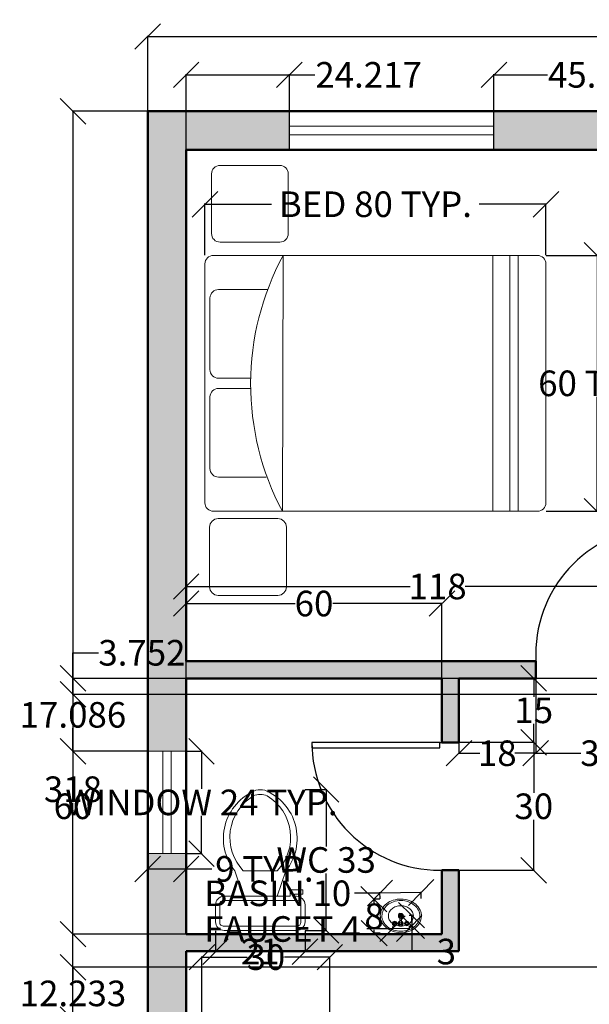
# Model space of a CAD drawing. Units: inches. Extents: x -29 to 284, y -310 to 51.
# Tile 2 of 4: x -29 to 105, y -180 to 51. Entities that reach past the tile are written whole.
import ezdxf

# ---------------------------------------------------------------- set-up
doc = ezdxf.new("R2010")
doc.units = ezdxf.units.IN
doc.header["$MEASUREMENT"] = 0
for name, color, linetype, lineweight in [('A-ANNO-DIMS', 2, 'Continuous', 18), ('A-DOOR', 3, 'Continuous', 25), ('A-FLOR-FIXT', 9, 'Continuous', 18), ('A-FURN', 8, 'Continuous', 18), ('A-GLAZ', 4, 'Continuous', 18), ('A-WALL', 7, 'Continuous', 50)]:
    doc.layers.add(name, color=color, linetype=linetype, lineweight=lineweight)
doc.layers.add('A-WALL-PATT', color=18, linetype='Continuous', lineweight=13, true_color=0x000000)
doc.styles.get("Standard").update_dxf_attribs({"font": 'arial.ttf'})
doc.dimstyles.get("Standard").update_dxf_attribs({"dimtxt": 6, "dimasz": 6, "dimexe": 0.18, "dimexo": 0.0625, "dimgap": 0.09, "dimtad": 0, "dimtih": 1, "dimtoh": 1, "dimdec": 0, "dimzin": 0, "dimdsep": 46, "dimlunit": 4, "dimtxsty": 'Standard', "dimblk": 'OBLIQUE', "dimcen": 0.09, "dimadec": 0, "dimazin": 0, "dimtfac": 1, "dimtdec": 0, "dimtofl": 0, "dimtmove": 0, "dimatfit": 3, "dimldrblk": 'OBLIQUE', "dimfxl": 1, "dimtolj": 1, "dimtzin": 0, "dimarcsym": 0})

# ---------------------------------------------------------------- blocks, each defined once
blk = doc.blocks.new('Bed - Queen')
for p, q in [((2, 0), (58, 0)), ((0, -78), (0, -2)), ((10, -1.2), (26.8, -1.2)), ((33.2, -1.2), (50, -1.2)), ((60, -2), (60, -78)), ((8, -14.4), (8, -3.2)), ((28.8, -3.2), (28.8, -10.75)), ((31.2, -10.81), (31.2, -3.2)), ((52, -3.2), (52, -14.74)), ((0, -18.19), (60, -18.37)), ((0, -67.53), (60, -67.53)), ((0, -71.53), (60, -71.53)), ((0, -73.53), (60, -73.53)), ((58, -80), (2, -80))]:
    blk.add_line(p, q)
for centre, radius, start, end in [((2, -2), 2, 90, 180), ((58, -2), 2, 0, 90), ((10, -3.2), 2, 90, 180), ((26.8, -3.2), 2, 0, 90), ((33.2, -3.2), 2, 90, 180), ((50, -3.2), 2, 0, 90), ((29.83, -74.22), 63.48, 61.626, 118.0335), ((2, -78), 2, 180, 270), ((58, -78), 2, 270, 0)]:
    blk.add_arc(centre, radius, start, end)
blk = doc.blocks.new('Toilet - top')
for p, q in [((9.5, -6), (9.5, -2)), ((-10, -8.5), (-8, -8.5)), ((-10, -9.5), (-10, -8.5)), ((-8, -8.5), (-8, -8)), ((-7, -8), (-7, -9.5)), ((-4, -8), (-6, -14)), ((4, -8), (6, -14)), ((-7, -9.5), (-10, -9.5)), ((4, -14), (-4, -14))]:
    blk.add_line(p, q)
blk.add_lwpolyline([(-7, -8), (8.5, -8, 0.414214), (10.5, -6), (10.5, -2, 0.414214), (8.5, 0), (-8.5, 0, 0.414214), (-10.5, -2), (-10.5, -6, 0.414214), (-8.5, -8), (-8, -8)], format="xyb")
for points in [[(-9.5, -2), (-9.5, -6)], [(8.5, -1), (-8.5, -1)], [(-8.5, -7), (8.5, -7)]]:
    blk.add_lwpolyline(points)
for centre, radius, start, end in [((-8.62, -1.88), 0.884, 81.8699, 188.1301), ((8.62, -1.88), 0.884, 351.8699, 98.1301), ((-8.62, -6.12), 0.884, 171.8699, 278.1301), ((8.62, -6.12), 0.884, 261.8699, 8.1301), ((3.52, -21.58), 12.17, 141.4691, 247.9714), ((4.2, -21.82), 11.33, 136.3677, 238.9468), ((-3.52, -21.58), 12.17, 292.0284, 38.5307), ((-4.2, -21.82), 11.33, 301.053, 43.6321), ((0, -27.88), 4, 245.7318, 294.2682), ((0, -29), 4, 254.8605, 285.1395)]:
    blk.add_arc(centre, radius, start, end)
blk = doc.blocks.new('Sink - Oval top')
for p, q in [((-1, 0), (1, 0)), ((0, 1), (0, -1))]:
    blk.add_line(p, q)
for points in [[(-12.23, 0.39, 0.117634), (-11.46, -3.36, 0.104469), (-8.88, -6.8, 0.090016), (-5.08, -9.07, 0.08192), (-0.32, -10.02, 0.08192), (4.49, -9.38, 0.090016), (8.42, -7.36, 0.104469), (11.22, -4.09, 0.117634), (12.23, -0.39, 0.117634), (11.46, 3.36, 0.104469), (8.88, 6.8, 0.090016), (5.08, 9.07, 0.08192), (0.32, 10.02, 0.08192), (-4.49, 9.38, 0.090016), (-8.42, 7.36, 0.104469), (-11.22, 4.09, 0.117634)], [(-11.29, 0.16, 0.118622), (-10.52, -3.25, 0.104678), (-8.07, -6.36, 0.089562), (-4.54, -8.37, 0.081185), (-0.13, -9.15, 0.081185), (4.3, -8.49, 0.089562), (7.89, -6.58, 0.104678), (10.42, -3.55, 0.118622), (11.29, -0.16, 0.118622), (10.52, 3.25, 0.104678), (8.07, 6.36, 0.089562), (4.54, 8.37, 0.081185), (0.13, 9.15, 0.081185), (-4.3, 8.49, 0.089562), (-7.89, 6.58, 0.104678), (-10.42, 3.55, 0.118622)], [(-7.42, 0.08, 0.118283), (-6.91, -2.17, 0.104607), (-5.29, -4.21, 0.089718), (-2.97, -5.53, 0.081436), (-0.07, -6.04, 0.081436), (2.84, -5.59, 0.089718), (5.2, -4.33, 0.104607), (6.86, -2.32, 0.118283), (7.42, -0.08, 0.118283), (6.91, 2.17, 0.104607), (5.29, 4.21, 0.089718), (2.97, 5.53, 0.081436), (0.07, 6.04, 0.081436), (-2.84, 5.59, 0.089718), (-5.2, 4.33, 0.104607), (-6.86, 2.32, 0.118283)]]:
    blk.add_lwpolyline(points, format="xyb", close=True)
for radius in [1.5, 1]:
    blk.add_circle((0, 0), radius)
blk = doc.blocks.new('Faucet - Bathroom top')
for p, q in [((-4.107, 0.125), (-4.375, 0.125)), ((-3.75, 0.4788), (-3.75, 0.75)), ((-3.5, 0.482), (-3.5, 0.75)), ((-3.1461, 0.125), (-2.875, 0.125)), ((3.143, 0.125), (2.875, 0.125)), ((3.5, 0.4788), (3.5, 0.75)), ((3.75, 0.482), (3.75, 0.75)), ((4.1039, 0.125), (4.375, 0.125)), ((-4.1039, -0.125), (-4.375, -0.125)), ((-3.75, -0.4821), (-3.75, -0.75)), ((-3.5, -0.4789), (-3.5, -0.75)), ((-3.143, -0.125), (-2.875, -0.125)), ((-0.5, -0.8639), (-0.5, -4.5)), ((0.5, -4.5), (0.5, -0.8631)), ((3.1461, -0.125), (2.875, -0.125)), ((3.5, -0.4821), (3.5, -0.75)), ((3.75, -0.4789), (3.75, -0.75)), ((4.107, -0.125), (4.375, -0.125))]:
    blk.add_line(p, q)
for centre, radius in [((-3.625, 0), 1.375), ((-4.625, 0), 0.2795), ((-3.625, 0), 0.5), ((-3.625, 1), 0.2795), ((-2.625, 0), 0.2795), ((0, 0), 0.5), ((3.625, 0), 1.375), ((2.625, 0), 0.2795), ((3.625, 0), 0.5), ((3.625, 1), 0.2795), ((4.625, 0), 0.2795), ((-3.625, -1), 0.2795), ((3.625, -1), 0.2795)]:
    blk.add_circle(centre, radius)
for centre, radius, start, end in [((-3.625, 0), 1, 105.2407, 164.2093), ((-3.625, 0), 1, 16.44125, 74.07887), ((0, 0), 1.5, 289.6514, 250.3603), ((0, 0), 1, 300.3431, 239.7554), ((3.625, 0), 1, 106.12, 164.0884), ((3.625, 0), 1, 16.23422, 73.90469), ((-3.625, 0), 1, 196.2342, 253.9047), ((-3.625, 0), 1, 286.12, 344.0884), ((0, -4.5), 0.5, 180, 0), ((3.625, 0), 1, 196.4413, 254.0789), ((3.625, 0), 1, 285.2407, 344.2093)]:
    blk.add_arc(centre, radius, start, end)
blk = doc.blocks.new('*U14')
for p, q in [((0, 0), (0, -6)), ((-40, 0), (-40, -6))]:
    blk.add_line(p, q)
blk.add_lwpolyline([(0, 0), (0, 40), (-1.75, 40), (-1.75, 0)], close=True)
blk.add_arc((0, 0), 40, 90, 180)
blk = doc.blocks.new('*U15')
for p, q in [((0, 0), (0, 6)), ((40, 0), (40, 6))]:
    blk.add_line(p, q)
blk.add_lwpolyline([(0, 0), (0, -40), (1.75, -40), (1.75, 0)], close=True)
blk.add_arc((0, 0), 40, 270, 0)
blk = doc.blocks.new('WIN-48IN')
for p, q in [((0, 5.5), (48, 5.5)), ((0, 3.5), (48, 3.5))]:
    blk.add_line(p, q)
for points in [[(0, 0), (0, 9)], [(48, 9), (48, 0)]]:
    blk.add_lwpolyline(points)
blk = doc.blocks.new('WIN-24IN')
for p, q in [((3.5, 24), (3.5, 0)), ((5.5, 24), (5.5, 0))]:
    blk.add_line(p, q)
for points in [[(0, 24), (9, 24)], [(9, 0), (0, 0)]]:
    blk.add_lwpolyline(points)
blk = doc.blocks.new('NIGHTSTAND-18IN')
blk.add_lwpolyline([(0, 2), (0, 16, -0.414214), (2, 18), (16, 18, -0.414214), (18, 16), (18, 2, -0.414214), (16, 0), (2, 0, -0.414214)], format="xyb", close=True)
blk = doc.blocks.new('_Oblique')
at = {"color": 0, "linetype": 'ByBlock', "lineweight": -2}
blk.add_line((-0.5, -0.5), (0.5, 0.5), dxfattribs=at)
blk = doc.blocks.new('*D25')
at = {"layer": 'A-ANNO-DIMS', "color": 0, "lineweight": -2, "transparency": 16777216}
for p, q in [((14.38, -4.3), (14.38, 7.82)), ((14.38, 7.64), (30.04, 7.64)), ((94.38, 7.64), (78.72, 7.64)), ((94.38, -4.3), (94.38, 7.82))]:
    blk.add_line(p, q, dxfattribs=at)
at = {"layer": 'Defpoints', "color": 0, "transparency": 16777216}
for p in [(14.38, 7.64), (14.38, -4.36), (94.38, -4.36)]:
    blk.add_point(p, dxfattribs=at)
at = {"layer": 'A-ANNO-DIMS', "color": 0, "lineweight": -2, "transparency": 16777216, "xscale": 6, "yscale": 6, "zscale": 6, "rotation": 180}
blk.add_blockref('_Oblique', (14.38, 7.64), dxfattribs=at)
at = {"layer": 'A-ANNO-DIMS', "color": 0, "lineweight": -2, "transparency": 16777216, "xscale": 6, "yscale": 6, "zscale": 6}
blk.add_blockref('_Oblique', (94.38, 7.64), dxfattribs=at)
at = {"layer": 'A-ANNO-DIMS', "color": 0, "transparency": 16777216, "insert": (54.38, 7.64), "char_height": 6, "attachment_point": 5}
blk.add_mtext('\\A1;BED 80 TYP.', dxfattribs=at)
blk = doc.blocks.new('*D26')
at = {"layer": 'A-ANNO-DIMS', "color": 0, "lineweight": -2, "transparency": 16777216}
for p, q in [((94.44, -4.36), (106.56, -4.36)), ((106.38, -4.36), (106.38, -31.2)), ((106.38, -64.36), (106.38, -37.51)), ((94.44, -64.36), (106.56, -64.36))]:
    blk.add_line(p, q, dxfattribs=at)
at = {"layer": 'Defpoints', "color": 0, "transparency": 16777216}
for p in [(94.38, -4.36), (106.38, -4.36), (94.38, -64.36)]:
    blk.add_point(p, dxfattribs=at)
at = {"layer": 'A-ANNO-DIMS', "color": 0, "lineweight": -2, "transparency": 16777216, "xscale": 6, "yscale": 6, "zscale": 6}
for p, rotation in [((106.38, -4.36), 90), ((106.38, -64.36), 270)]:
    blk.add_blockref('_Oblique', p, dxfattribs=dict(at, rotation=rotation))
at = {"layer": 'A-ANNO-DIMS', "color": 0, "transparency": 16777216, "insert": (106.38, -34.36), "char_height": 6, "attachment_point": 5}
blk.add_mtext('\\A1;60 TYP.', dxfattribs=at)
blk = doc.blocks.new('*D29')
at = {"layer": 'A-ANNO-DIMS', "color": 0, "lineweight": -2, "transparency": 16777216}
for p, q in [((10.04, -120.65), (13.76, -120.65)), ((13.58, -120.65), (13.58, -129.46)), ((13.58, -144.65), (13.58, -135.84)), ((10.04, -144.65), (13.76, -144.65))]:
    blk.add_line(p, q, dxfattribs=at)
at = {"layer": 'Defpoints', "color": 0, "transparency": 16777216}
for p in [(9.98, -120.65), (13.58, -120.65), (9.98, -144.65)]:
    blk.add_point(p, dxfattribs=at)
at = {"layer": 'A-ANNO-DIMS', "color": 0, "lineweight": -2, "transparency": 16777216, "xscale": 6, "yscale": 6, "zscale": 6}
for p, rotation in [((13.58, -120.65), 90), ((13.58, -144.65), 270)]:
    blk.add_blockref('_Oblique', p, dxfattribs=dict(at, rotation=rotation))
at = {"layer": 'A-ANNO-DIMS', "color": 0, "transparency": 16777216, "insert": (13.58, -132.65), "char_height": 6, "attachment_point": 5}
blk.add_mtext('\\A1;WINDOW 24 TYP.', dxfattribs=at)
blk = doc.blocks.new('*D30')
at = {"layer": 'A-ANNO-DIMS', "color": 0, "lineweight": -2, "transparency": 16777216}
for p, q in [((0.98, -144.71), (0.98, -148.43)), ((9.98, -144.71), (9.98, -148.43)), ((0.98, -148.25), (9.98, -148.25)), ((9.98, -148.25), (15.98, -148.25))]:
    blk.add_line(p, q, dxfattribs=at)
at = {"layer": 'Defpoints', "color": 0, "transparency": 16777216}
for p in [(0.98, -144.65), (9.98, -144.65), (9.98, -148.25)]:
    blk.add_point(p, dxfattribs=at)
at = {"layer": 'A-ANNO-DIMS', "color": 0, "lineweight": -2, "transparency": 16777216, "xscale": 6, "yscale": 6, "zscale": 6, "rotation": 180}
blk.add_blockref('_Oblique', (0.98, -148.25), dxfattribs=at)
at = {"layer": 'A-ANNO-DIMS', "color": 0, "lineweight": -2, "transparency": 16777216, "xscale": 6, "yscale": 6, "zscale": 6}
blk.add_blockref('_Oblique', (9.98, -148.25), dxfattribs=at)
at = {"layer": 'A-ANNO-DIMS', "color": 0, "transparency": 16777216, "insert": (28.34, -148.25), "char_height": 6, "attachment_point": 5}
blk.add_mtext('\\A1;9 TYP.', dxfattribs=at)
blk = doc.blocks.new('*D39')
at = {"layer": 'A-ANNO-DIMS', "color": 0, "lineweight": -2, "transparency": 16777216}
for p, q in [((37.94, -129.63), (43.01, -129.63)), ((42.83, -129.63), (42.83, -142.96)), ((42.83, -162.67), (42.83, -149.35)), ((37.94, -162.67), (43.01, -162.67))]:
    blk.add_line(p, q, dxfattribs=at)
at = {"layer": 'Defpoints', "color": 0, "transparency": 16777216}
for p in [(37.88, -129.63), (37.88, -162.67), (42.83, -162.67)]:
    blk.add_point(p, dxfattribs=at)
at = {"layer": 'A-ANNO-DIMS', "color": 0, "lineweight": -2, "transparency": 16777216, "xscale": 6, "yscale": 6, "zscale": 6}
for p, rotation in [((42.83, -129.63), 90), ((42.83, -162.67), 270)]:
    blk.add_blockref('_Oblique', p, dxfattribs=dict(at, rotation=rotation))
at = {"layer": 'A-ANNO-DIMS', "color": 0, "transparency": 16777216, "insert": (42.83, -146.15), "char_height": 6, "attachment_point": 5}
blk.add_mtext('\\A1;WC 33', dxfattribs=at)
blk = doc.blocks.new('*D40')
at = {"layer": 'A-ANNO-DIMS', "color": 0, "lineweight": -2, "transparency": 16777216}
for p, q in [((16.88, -162.74), (16.88, -167.81)), ((37.88, -162.74), (37.88, -167.81)), ((16.88, -167.63), (23.52, -167.63)), ((37.88, -167.63), (31.24, -167.63))]:
    blk.add_line(p, q, dxfattribs=at)
at = {"layer": 'Defpoints', "color": 0, "transparency": 16777216}
for p in [(16.88, -162.67), (37.88, -162.67), (16.88, -167.63)]:
    blk.add_point(p, dxfattribs=at)
at = {"layer": 'A-ANNO-DIMS', "color": 0, "lineweight": -2, "transparency": 16777216, "xscale": 6, "yscale": 6, "zscale": 6, "rotation": 180}
blk.add_blockref('_Oblique', (16.88, -167.63), dxfattribs=at)
at = {"layer": 'A-ANNO-DIMS', "color": 0, "lineweight": -2, "transparency": 16777216, "xscale": 6, "yscale": 6, "zscale": 6}
blk.add_blockref('_Oblique', (37.88, -167.63), dxfattribs=at)
at = {"layer": 'A-ANNO-DIMS', "color": 0, "transparency": 16777216, "insert": (27.38, -167.63), "char_height": 6, "attachment_point": 5}
blk.add_mtext('\\A1;21', dxfattribs=at)
blk = doc.blocks.new('*D41')
at = {"layer": 'A-ANNO-DIMS', "color": 0, "lineweight": -2, "transparency": 16777216}
for p, q in [((55.46, -153.91), (49.46, -153.97)), ((55.48, -155.29), (55.46, -153.73)), ((65.14, -153.8), (55.46, -153.91)), ((65.15, -155.19), (65.14, -153.62))]:
    blk.add_line(p, q, dxfattribs=at)
at = {"layer": 'Defpoints', "color": 0, "transparency": 16777216}
for p in [(55.46, -153.91), (55.48, -155.36), (65.15, -155.25)]:
    blk.add_point(p, dxfattribs=at)
at = {"layer": 'A-ANNO-DIMS', "color": 0, "lineweight": -2, "transparency": 16777216, "xscale": 6, "yscale": 6, "zscale": 6}
for p, rotation in [((55.46, -153.91), 180.628378081795), ((65.14, -153.8), 0.6283780817949493)]:
    blk.add_blockref('_Oblique', p, dxfattribs=dict(at, rotation=rotation))
at = {"layer": 'A-ANNO-DIMS', "color": 0, "transparency": 16777216, "insert": (31.48, -153.97), "char_height": 6, "attachment_point": 5}
blk.add_mtext('\\A1;BASIN 10', dxfattribs=at)
blk = doc.blocks.new('*D42')
at = {"layer": 'A-ANNO-DIMS', "color": 0, "lineweight": -2, "transparency": 16777216}
for p, q in [((55.42, -155.36), (53.85, -155.38)), ((54.03, -155.37), (54.04, -156.19)), ((55.5, -163.29), (53.93, -163.31)), ((54.11, -163.31), (54.1, -162.5))]:
    blk.add_line(p, q, dxfattribs=at)
at = {"layer": 'Defpoints', "color": 0, "transparency": 16777216}
for p in [(55.48, -155.36), (54.11, -163.31), (55.57, -163.29)]:
    blk.add_point(p, dxfattribs=at)
at = {"layer": 'A-ANNO-DIMS', "color": 0, "lineweight": -2, "transparency": 16777216, "xscale": 6, "yscale": 6, "zscale": 6}
for p, rotation in [((54.03, -155.37), 90.62837808179486), ((54.11, -163.31), 270.6283780817949)]:
    blk.add_blockref('_Oblique', p, dxfattribs=dict(at, rotation=rotation))
at = {"layer": 'A-ANNO-DIMS', "color": 0, "transparency": 16777216, "insert": (54.07, -159.34), "char_height": 6, "attachment_point": 5}
blk.add_mtext('\\A1;8', dxfattribs=at)
blk = doc.blocks.new('*D43')
at = {"layer": 'A-ANNO-DIMS', "color": 0, "lineweight": -2, "transparency": 16777216}
for p, q in [((58.37, -162.27), (52.37, -162.34)), ((58.36, -161.74), (58.37, -162.45)), ((62.31, -162.23), (58.37, -162.27)), ((62.3, -161.7), (62.31, -162.41))]:
    blk.add_line(p, q, dxfattribs=at)
at = {"layer": 'Defpoints', "color": 0, "transparency": 16777216}
for p in [(62.3, -161.63), (58.36, -161.68), (58.37, -162.27)]:
    blk.add_point(p, dxfattribs=at)
at = {"layer": 'A-ANNO-DIMS', "color": 0, "lineweight": -2, "transparency": 16777216, "xscale": 6, "yscale": 6, "zscale": 6}
for p, rotation in [((58.37, -162.27), 180.6283780817947), ((62.31, -162.23), 0.6283780817947893)]:
    blk.add_blockref('_Oblique', p, dxfattribs=dict(at, rotation=rotation))
at = {"layer": 'A-ANNO-DIMS', "color": 0, "transparency": 16777216, "insert": (32.57, -162.34), "char_height": 6, "attachment_point": 5}
blk.add_mtext('\\A1;FAUCET 4', dxfattribs=at)
blk = doc.blocks.new('*D44')
at = {"layer": 'A-ANNO-DIMS', "color": 0, "lineweight": -2, "transparency": 16777216}
for p, q in [((62.34, -159.07), (63.05, -159.06)), ((62.87, -159.07), (62.9, -161.63)), ((62.37, -161.63), (63.08, -161.63)), ((62.9, -161.63), (62.96, -167.63)), ((62.96, -167.63), (68.96, -167.63))]:
    blk.add_line(p, q, dxfattribs=at)
at = {"layer": 'Defpoints', "color": 0, "transparency": 16777216}
for p in [(62.28, -159.07), (62.3, -161.63), (62.9, -161.63)]:
    blk.add_point(p, dxfattribs=at)
at = {"layer": 'A-ANNO-DIMS', "color": 0, "lineweight": -2, "transparency": 16777216, "xscale": 6, "yscale": 6, "zscale": 6}
for p, rotation in [((62.87, -159.07), 90.62837808179493), ((62.9, -161.63), 270.6283780817949)]:
    blk.add_blockref('_Oblique', p, dxfattribs=dict(at, rotation=rotation))
at = {"layer": 'A-ANNO-DIMS', "color": 0, "transparency": 16777216, "insert": (71.02, -167.63), "char_height": 6, "attachment_point": 5}
blk.add_mtext('\\A1;3', dxfattribs=at)
blk = doc.blocks.new('*D45')
at = {"layer": 'A-ANNO-DIMS', "color": 0, "lineweight": -2, "transparency": 16777216}
for p, q in [((0.98, 29.5), (0.98, 47.17)), ((0.98, 46.99), (123.21, 46.99)), ((258.98, 46.99), (136.76, 46.99)), ((258.98, 29.5), (258.98, 47.17))]:
    blk.add_line(p, q, dxfattribs=at)
at = {"layer": 'Defpoints', "color": 0, "transparency": 16777216}
for p in [(258.98, 46.99), (0.98, 29.44), (258.98, 29.44)]:
    blk.add_point(p, dxfattribs=at)
at = {"layer": 'A-ANNO-DIMS', "color": 0, "lineweight": -2, "transparency": 16777216, "xscale": 6, "yscale": 6, "zscale": 6, "rotation": 180}
blk.add_blockref('_Oblique', (0.98, 46.99), dxfattribs=at)
at = {"layer": 'A-ANNO-DIMS', "color": 0, "lineweight": -2, "transparency": 16777216, "xscale": 6, "yscale": 6, "zscale": 6}
blk.add_blockref('_Oblique', (258.98, 46.99), dxfattribs=at)
at = {"layer": 'A-ANNO-DIMS', "color": 0, "transparency": 16777216, "insert": (129.98, 46.99), "char_height": 6, "attachment_point": 5}
blk.add_mtext('\\A1;258', dxfattribs=at)
blk = doc.blocks.new('*D46')
at = {"layer": 'A-ANNO-DIMS', "color": 0, "lineweight": -2, "transparency": 16777216}
for p, q in [((0.92, 29.44), (-16.75, 29.44)), ((-16.57, 29.44), (-16.57, -126.41)), ((-16.57, -288.56), (-16.57, -132.72)), ((0.92, -288.56), (-16.75, -288.56))]:
    blk.add_line(p, q, dxfattribs=at)
at = {"layer": 'Defpoints', "color": 0, "transparency": 16777216}
for p in [(-16.57, 29.44), (0.98, 29.44), (0.98, -288.56)]:
    blk.add_point(p, dxfattribs=at)
at = {"layer": 'A-ANNO-DIMS', "color": 0, "lineweight": -2, "transparency": 16777216, "xscale": 6, "yscale": 6, "zscale": 6}
for p, rotation in [((-16.57, 29.44), 90), ((-16.57, -288.56), 270)]:
    blk.add_blockref('_Oblique', p, dxfattribs=dict(at, rotation=rotation))
at = {"layer": 'A-ANNO-DIMS', "color": 0, "transparency": 16777216, "insert": (-16.57, -129.56), "char_height": 6, "attachment_point": 5}
blk.add_mtext('\\A1;318', dxfattribs=at)
blk = doc.blocks.new('*D47')
at = {"layer": 'A-ANNO-DIMS', "color": 0, "lineweight": -2, "transparency": 16777216}
for p, q in [((9.98, 20.5), (9.98, 38.17)), ((9.98, 37.99), (34.2, 37.99)), ((34.2, 20.5), (34.2, 38.17)), ((34.2, 37.99), (40.2, 37.99))]:
    blk.add_line(p, q, dxfattribs=at)
at = {"layer": 'Defpoints', "color": 0, "transparency": 16777216}
for p in [(34.2, 37.99), (9.98, 20.44), (34.2, 20.44)]:
    blk.add_point(p, dxfattribs=at)
at = {"layer": 'A-ANNO-DIMS', "color": 0, "lineweight": -2, "transparency": 16777216, "xscale": 6, "yscale": 6, "zscale": 6, "rotation": 180}
blk.add_blockref('_Oblique', (9.98, 37.99), dxfattribs=at)
at = {"layer": 'A-ANNO-DIMS', "color": 0, "lineweight": -2, "transparency": 16777216, "xscale": 6, "yscale": 6, "zscale": 6}
blk.add_blockref('_Oblique', (34.2, 37.99), dxfattribs=at)
at = {"layer": 'A-ANNO-DIMS', "color": 0, "transparency": 16777216, "insert": (52.79, 37.99), "char_height": 6, "attachment_point": 5}
blk.add_mtext('\\A1;24.217', dxfattribs=at)
blk = doc.blocks.new('*D48')
at = {"layer": 'A-ANNO-DIMS', "color": 0, "lineweight": -2, "transparency": 16777216}
for p, q in [((82.2, 20.5), (82.2, 38.17)), ((82.2, 37.99), (94.75, 37.99)), ((127.98, 37.99), (115.43, 37.99)), ((127.98, 20.5), (127.98, 38.17))]:
    blk.add_line(p, q, dxfattribs=at)
at = {"layer": 'Defpoints', "color": 0, "transparency": 16777216}
for p in [(127.98, 37.99), (82.2, 20.44), (127.98, 20.44)]:
    blk.add_point(p, dxfattribs=at)
at = {"layer": 'A-ANNO-DIMS', "color": 0, "lineweight": -2, "transparency": 16777216, "xscale": 6, "yscale": 6, "zscale": 6, "rotation": 180}
blk.add_blockref('_Oblique', (82.2, 37.99), dxfattribs=at)
at = {"layer": 'A-ANNO-DIMS', "color": 0, "lineweight": -2, "transparency": 16777216, "xscale": 6, "yscale": 6, "zscale": 6}
blk.add_blockref('_Oblique', (127.98, 37.99), dxfattribs=at)
at = {"layer": 'A-ANNO-DIMS', "color": 0, "transparency": 16777216, "insert": (105.09, 37.99), "char_height": 6, "attachment_point": 5}
blk.add_mtext('\\A1;45.78', dxfattribs=at)
blk = doc.blocks.new('*D52')
at = {"layer": 'A-ANNO-DIMS', "color": 0, "lineweight": -2, "transparency": 16777216}
for p, q in [((9.98, -99.5), (9.98, -81.83)), ((9.98, -82.01), (62.54, -82.01)), ((127.98, -82.01), (75.42, -82.01)), ((127.98, -99.5), (127.98, -81.83))]:
    blk.add_line(p, q, dxfattribs=at)
at = {"layer": 'Defpoints', "color": 0, "transparency": 16777216}
for p in [(127.98, -82.01), (9.98, -99.56), (127.98, -99.56)]:
    blk.add_point(p, dxfattribs=at)
at = {"layer": 'A-ANNO-DIMS', "color": 0, "lineweight": -2, "transparency": 16777216, "xscale": 6, "yscale": 6, "zscale": 6, "rotation": 180}
blk.add_blockref('_Oblique', (9.98, -82.01), dxfattribs=at)
at = {"layer": 'A-ANNO-DIMS', "color": 0, "lineweight": -2, "transparency": 16777216, "xscale": 6, "yscale": 6, "zscale": 6}
blk.add_blockref('_Oblique', (127.98, -82.01), dxfattribs=at)
at = {"layer": 'A-ANNO-DIMS', "color": 0, "transparency": 16777216, "insert": (68.98, -82.01), "char_height": 6, "attachment_point": 5}
blk.add_mtext('\\A1;118', dxfattribs=at)
blk = doc.blocks.new('*D54')
at = {"layer": 'A-ANNO-DIMS', "color": 0, "lineweight": -2, "transparency": 16777216}
for p, q in [((73.98, -103.63), (73.98, -121.29)), ((91.98, -103.63), (91.98, -121.29)), ((73.98, -121.11), (78.87, -121.11)), ((91.98, -121.11), (87.09, -121.11))]:
    blk.add_line(p, q, dxfattribs=at)
at = {"layer": 'Defpoints', "color": 0, "transparency": 16777216}
for p in [(73.98, -103.56), (91.98, -103.56), (73.98, -121.11)]:
    blk.add_point(p, dxfattribs=at)
at = {"layer": 'A-ANNO-DIMS', "color": 0, "lineweight": -2, "transparency": 16777216, "xscale": 6, "yscale": 6, "zscale": 6, "rotation": 180}
blk.add_blockref('_Oblique', (73.98, -121.11), dxfattribs=at)
at = {"layer": 'A-ANNO-DIMS', "color": 0, "lineweight": -2, "transparency": 16777216, "xscale": 6, "yscale": 6, "zscale": 6}
blk.add_blockref('_Oblique', (91.98, -121.11), dxfattribs=at)
at = {"layer": 'A-ANNO-DIMS', "color": 0, "transparency": 16777216, "insert": (82.98, -121.11), "char_height": 6, "attachment_point": 5}
blk.add_mtext('\\A1;18', dxfattribs=at)
blk = doc.blocks.new('*D55')
at = {"layer": 'A-ANNO-DIMS', "color": 0, "lineweight": -2, "transparency": 16777216}
for p, q in [((91.98, -103.63), (91.98, -121.29)), ((121.98, -103.63), (121.98, -121.29)), ((91.98, -121.11), (102.61, -121.11)), ((121.98, -121.11), (111.36, -121.11))]:
    blk.add_line(p, q, dxfattribs=at)
at = {"layer": 'Defpoints', "color": 0, "transparency": 16777216}
for p in [(91.98, -103.56), (121.98, -103.56), (91.98, -121.11)]:
    blk.add_point(p, dxfattribs=at)
at = {"layer": 'A-ANNO-DIMS', "color": 0, "lineweight": -2, "transparency": 16777216, "xscale": 6, "yscale": 6, "zscale": 6, "rotation": 180}
blk.add_blockref('_Oblique', (91.98, -121.11), dxfattribs=at)
at = {"layer": 'A-ANNO-DIMS', "color": 0, "lineweight": -2, "transparency": 16777216, "xscale": 6, "yscale": 6, "zscale": 6}
blk.add_blockref('_Oblique', (121.98, -121.11), dxfattribs=at)
at = {"layer": 'A-ANNO-DIMS', "color": 0, "transparency": 16777216, "insert": (106.98, -121.11), "char_height": 6, "attachment_point": 5}
blk.add_mtext('\\A1;30', dxfattribs=at)
blk = doc.blocks.new('*D58')
at = {"layer": 'A-ANNO-DIMS', "color": 0, "lineweight": -2, "transparency": 16777216}
for p, q in [((9.98, -103.5), (9.98, -85.83)), ((9.98, -86.01), (35.59, -86.01)), ((69.98, -86.01), (44.37, -86.01)), ((69.98, -103.5), (69.98, -85.83))]:
    blk.add_line(p, q, dxfattribs=at)
at = {"layer": 'Defpoints', "color": 0, "transparency": 16777216}
for p in [(69.98, -86.01), (9.98, -103.56), (69.98, -103.56)]:
    blk.add_point(p, dxfattribs=at)
at = {"layer": 'A-ANNO-DIMS', "color": 0, "lineweight": -2, "transparency": 16777216, "xscale": 6, "yscale": 6, "zscale": 6, "rotation": 180}
blk.add_blockref('_Oblique', (9.98, -86.01), dxfattribs=at)
at = {"layer": 'A-ANNO-DIMS', "color": 0, "lineweight": -2, "transparency": 16777216, "xscale": 6, "yscale": 6, "zscale": 6}
blk.add_blockref('_Oblique', (69.98, -86.01), dxfattribs=at)
at = {"layer": 'A-ANNO-DIMS', "color": 0, "transparency": 16777216, "insert": (39.98, -86.01), "char_height": 6, "attachment_point": 5}
blk.add_mtext('\\A1;60', dxfattribs=at)
blk = doc.blocks.new('*D59')
at = {"layer": 'A-ANNO-DIMS', "color": 0, "lineweight": -2, "transparency": 16777216}
for p, q in [((9.92, -103.56), (-16.75, -103.56)), ((-16.57, -103.56), (-16.57, -130.41)), ((-16.57, -163.56), (-16.57, -136.72)), ((9.92, -163.56), (-16.75, -163.56))]:
    blk.add_line(p, q, dxfattribs=at)
at = {"layer": 'Defpoints', "color": 0, "transparency": 16777216}
for p in [(9.98, -103.56), (-16.57, -163.56), (9.98, -163.56)]:
    blk.add_point(p, dxfattribs=at)
at = {"layer": 'A-ANNO-DIMS', "color": 0, "lineweight": -2, "transparency": 16777216, "xscale": 6, "yscale": 6, "zscale": 6}
for p, rotation in [((-16.57, -103.56), 90), ((-16.57, -163.56), 270)]:
    blk.add_blockref('_Oblique', p, dxfattribs=dict(at, rotation=rotation))
at = {"layer": 'A-ANNO-DIMS', "color": 0, "transparency": 16777216, "insert": (-16.57, -133.56), "char_height": 6, "attachment_point": 5}
blk.add_mtext('\\A1;60', dxfattribs=at)
blk = doc.blocks.new('*D60')
at = {"layer": 'A-ANNO-DIMS', "color": 0, "lineweight": -2, "transparency": 16777216}
for p, q in [((74.04, -118.56), (91.71, -118.56)), ((91.53, -118.56), (91.53, -130.41)), ((91.53, -148.56), (91.53, -136.72)), ((74.04, -148.56), (91.71, -148.56))]:
    blk.add_line(p, q, dxfattribs=at)
at = {"layer": 'Defpoints', "color": 0, "transparency": 16777216}
for p in [(73.98, -118.56), (73.98, -148.56), (91.53, -148.56)]:
    blk.add_point(p, dxfattribs=at)
at = {"layer": 'A-ANNO-DIMS', "color": 0, "lineweight": -2, "transparency": 16777216, "xscale": 6, "yscale": 6, "zscale": 6}
for p, rotation in [((91.53, -118.56), 90), ((91.53, -148.56), 270)]:
    blk.add_blockref('_Oblique', p, dxfattribs=dict(at, rotation=rotation))
at = {"layer": 'A-ANNO-DIMS', "color": 0, "transparency": 16777216, "insert": (91.53, -133.56), "char_height": 6, "attachment_point": 5}
blk.add_mtext('\\A1;30', dxfattribs=at)
blk = doc.blocks.new('*D61')
at = {"layer": 'A-ANNO-DIMS', "color": 0, "lineweight": -2, "transparency": 16777216}
for p, q in [((74.04, -103.56), (91.71, -103.56)), ((91.53, -103.56), (91.53, -107.91)), ((91.53, -118.56), (91.53, -114.22)), ((74.04, -118.56), (91.71, -118.56))]:
    blk.add_line(p, q, dxfattribs=at)
at = {"layer": 'Defpoints', "color": 0, "transparency": 16777216}
for p in [(73.98, -103.56), (73.98, -118.56), (91.53, -118.56)]:
    blk.add_point(p, dxfattribs=at)
at = {"layer": 'A-ANNO-DIMS', "color": 0, "lineweight": -2, "transparency": 16777216, "xscale": 6, "yscale": 6, "zscale": 6}
for p, rotation in [((91.53, -103.56), 90), ((91.53, -118.56), 270)]:
    blk.add_blockref('_Oblique', p, dxfattribs=dict(at, rotation=rotation))
at = {"layer": 'A-ANNO-DIMS', "color": 0, "transparency": 16777216, "insert": (91.53, -111.06), "char_height": 6, "attachment_point": 5}
blk.add_mtext('\\A1;15', dxfattribs=at)
blk = doc.blocks.new('*D62')
at = {"layer": 'A-ANNO-DIMS', "color": 0, "lineweight": -2, "transparency": 16777216}
for p, q in [((9.92, -103.56), (-16.75, -103.56)), ((-16.57, -103.56), (-16.57, -108.95)), ((-16.57, -120.65), (-16.57, -115.26)), ((0.92, -120.65), (-16.75, -120.65))]:
    blk.add_line(p, q, dxfattribs=at)
at = {"layer": 'Defpoints', "color": 0, "transparency": 16777216}
for p in [(-16.57, -103.56), (9.98, -103.56), (0.98, -120.65)]:
    blk.add_point(p, dxfattribs=at)
at = {"layer": 'A-ANNO-DIMS', "color": 0, "lineweight": -2, "transparency": 16777216, "xscale": 6, "yscale": 6, "zscale": 6}
for p, rotation in [((-16.57, -103.56), 90), ((-16.57, -120.65), 270)]:
    blk.add_blockref('_Oblique', p, dxfattribs=dict(at, rotation=rotation))
at = {"layer": 'A-ANNO-DIMS', "color": 0, "transparency": 16777216, "insert": (-16.57, -112.11), "char_height": 6, "attachment_point": 5}
blk.add_mtext('\\A1;17.086', dxfattribs=at)
blk = doc.blocks.new('*D66')
at = {"layer": 'A-ANNO-DIMS', "color": 0, "lineweight": -2, "transparency": 16777216}
for p, q in [((-16.57, -103.56), (-16.57, -97.56)), ((-16.57, -97.56), (-10.57, -97.56)), ((225.92, -103.56), (-16.75, -103.56)), ((-16.57, -107.32), (-16.57, -103.56)), ((229.03, -107.32), (-16.75, -107.32))]:
    blk.add_line(p, q, dxfattribs=at)
at = {"layer": 'Defpoints', "color": 0, "transparency": 16777216}
for p in [(-16.57, -103.56), (225.98, -103.56), (229.09, -107.32)]:
    blk.add_point(p, dxfattribs=at)
at = {"layer": 'A-ANNO-DIMS', "color": 0, "lineweight": -2, "transparency": 16777216, "xscale": 6, "yscale": 6, "zscale": 6}
for p, rotation in [((-16.57, -103.56), 90), ((-16.57, -107.32), 270)]:
    blk.add_blockref('_Oblique', p, dxfattribs=dict(at, rotation=rotation))
at = {"layer": 'A-ANNO-DIMS', "color": 0, "transparency": 16777216, "insert": (-0.39, -97.56), "char_height": 6, "attachment_point": 5}
blk.add_mtext('\\A1;3.752', dxfattribs=at)
blk = doc.blocks.new('*D67')
at = {"layer": 'A-ANNO-DIMS', "color": 0, "lineweight": -2, "transparency": 16777216}
for p, q in [((228.27, -171.33), (-16.75, -171.33)), ((-16.57, -171.33), (-16.57, -174.29)), ((-16.57, -183.56), (-16.57, -180.6)), ((225.92, -183.56), (-16.75, -183.56))]:
    blk.add_line(p, q, dxfattribs=at)
at = {"layer": 'Defpoints', "color": 0, "transparency": 16777216}
for p in [(228.33, -171.33), (-16.57, -183.56), (225.98, -183.56)]:
    blk.add_point(p, dxfattribs=at)
at = {"layer": 'A-ANNO-DIMS', "color": 0, "lineweight": -2, "transparency": 16777216, "xscale": 6, "yscale": 6, "zscale": 6}
for p, rotation in [((-16.57, -171.33), 90), ((-16.57, -183.56), 270)]:
    blk.add_blockref('_Oblique', p, dxfattribs=dict(at, rotation=rotation))
at = {"layer": 'A-ANNO-DIMS', "color": 0, "transparency": 16777216, "insert": (-16.57, -177.45), "char_height": 6, "attachment_point": 5}
blk.add_mtext('\\A1;12.233', dxfattribs=at)
blk = doc.blocks.new('*D80')
at = {"layer": 'A-ANNO-DIMS', "color": 0, "lineweight": -2, "transparency": 16777216}
for p, q in [((13.69, -186.43), (13.69, -168.76)), ((13.69, -168.94), (24.32, -168.94)), ((43.69, -168.94), (33.07, -168.94)), ((43.69, -186.43), (43.69, -168.76))]:
    blk.add_line(p, q, dxfattribs=at)
at = {"layer": 'Defpoints', "color": 0, "transparency": 16777216}
for p in [(43.69, -168.94), (13.69, -186.49), (43.69, -186.49)]:
    blk.add_point(p, dxfattribs=at)
at = {"layer": 'A-ANNO-DIMS', "color": 0, "lineweight": -2, "transparency": 16777216, "xscale": 6, "yscale": 6, "zscale": 6, "rotation": 180}
blk.add_blockref('_Oblique', (13.69, -168.94), dxfattribs=at)
at = {"layer": 'A-ANNO-DIMS', "color": 0, "lineweight": -2, "transparency": 16777216, "xscale": 6, "yscale": 6, "zscale": 6}
blk.add_blockref('_Oblique', (43.69, -168.94), dxfattribs=at)
at = {"layer": 'A-ANNO-DIMS', "color": 0, "transparency": 16777216, "insert": (28.69, -168.94), "char_height": 6, "attachment_point": 5}
blk.add_mtext('\\A1;30', dxfattribs=at)

msp = doc.modelspace()

# ---------------------------------------------------------------- hatches: boundary and pattern name
at = {"layer": 'A-WALL-PATT'}
h = msp.add_hatch(color=256, dxfattribs=at)
h.dxf.hatch_style = 1
h.paths.add_polyline_path([(34.1984, 29.4365), (0.9809, 29.4365), (0.9809, -120.6496), (9.9809, -120.6496), (9.9809, -103.5635), (69.9809, -103.5635), (69.9809, -118.5635), (73.9809, -118.5635), (73.9809, -103.5635), (91.9809, -103.5635), (91.9809, -99.5635), (9.9809, -99.5635), (9.9809, 20.4365), (34.1984, 20.4365)])
h = msp.add_hatch(color=256, dxfattribs=at)
h.dxf.hatch_style = 1
h.paths.add_polyline_path([(9.9809, -99.5635), (9.9809, 20.4365), (34.1984, 20.4365), (34.1984, 29.4365), (0.9809, 29.4365), (0.9809, -120.6496), (9.9809, -120.6496), (9.9809, -103.5635), (69.9809, -103.5635), (69.9809, -118.5635), (73.9809, -118.5635), (73.9809, -103.5635), (91.9809, -103.5635), (91.9809, -99.5635)])
h = msp.add_hatch(color=256, dxfattribs=at)
h.dxf.hatch_style = 1
h.paths.add_polyline_path([(172.6409, 20.4365), (172.6409, 29.4365), (82.1984, 29.4365), (82.1984, 20.4365), (127.9809, 20.4365), (127.9809, -99.5635), (121.9809, -99.5635), (121.9809, -103.5635), (127.9809, -103.5635), (137.9809, -103.5635), (137.9809, -99.5635), (131.9809, -99.5635), (131.9809, 20.4365)])
h = msp.add_hatch(color=256, dxfattribs=at)
h.dxf.hatch_style = 1
h.paths.add_polyline_path([(9.9809, -167.5635), (73.9809, -167.5635), (73.9809, -163.5635), (73.9809, -148.5635), (69.9809, -148.5635), (69.9809, -163.5635), (9.9809, -163.5635), (9.9809, -144.6496), (0.9809, -144.6496), (0.9809, -288.5635), (27.8543, -288.5635), (27.8543, -279.5635), (9.9809, -279.5635)])

# ---------------------------------------------------------------- linework, layer by layer
at = {"layer": 'A-WALL'}
for p, q in [((9.9809, 20.4365), (127.9809, 20.4365)), ((9.9809, -99.5635), (9.9809, 20.4365)), ((9.9809, -99.5635), (91.9809, -99.5635)), ((91.9809, -99.5635), (91.9809, -103.5635)), ((9.9809, -103.5635), (69.9809, -103.5635)), ((9.9809, -163.5635), (9.9809, -103.5635)), ((69.9809, -118.5635), (69.9809, -103.5635)), ((73.9809, -103.5635), (91.9809, -103.5635)), ((73.9809, -118.5635), (73.9809, -103.5635)), ((69.9809, -118.5635), (73.9809, -118.5635)), ((69.9809, -163.5635), (69.9809, -148.5635)), ((69.9809, -148.5635), (73.9809, -148.5635)), ((73.9809, -163.5635), (73.9809, -148.5635)), ((9.9809, -163.5635), (69.9809, -163.5635)), ((73.9809, -163.5635), (73.9809, -167.5635)), ((9.9809, -279.5635), (9.9809, -167.5635)), ((9.9809, -167.5635), (73.9809, -167.5635))]:
    msp.add_line(p, q, dxfattribs=at)
msp.add_lwpolyline([(99.9809, -288.5635), (0.9809, -288.5635), (0.9809, 29.4365), (258.9809, 29.4365), (258.9809, -288.5635), (135.9809, -288.5635)], dxfattribs=at)

# ---------------------------------------------------------------- block references
at = {"layer": 'A-DOOR', "xscale": 0.75, "yscale": 0.75, "zscale": 0.75}
msp.add_blockref('*U14', (121.9809, -97.9623), dxfattribs=at)
at = {"layer": 'A-DOOR', "xscale": 0.75, "yscale": 0.75, "zscale": 0.75, "rotation": 270}
msp.add_blockref('*U15', (69.4809, -118.5635), dxfattribs=at)
at = {"layer": 'A-FLOR-FIXT', "rotation": 180}
msp.add_blockref('Toilet - top', (27.3756, -162.6741), dxfattribs=at)
at = {"layer": 'A-FLOR-FIXT', "xscale": 0.3941738778981024, "yscale": 0.3941738778981024, "zscale": 0.3941738778981024, "rotation": 180.6283780817949}
for name, p in [('Sink - Oval top', (60.3599, -159.2726)), ('Faucet - Bathroom top', (60.3268, -161.0653))]:
    msp.add_blockref(name, p, dxfattribs=at)
at = {"layer": 'A-FURN'}
for p in [(15.941, -1.248), (15.499, -84.0917)]:
    msp.add_blockref('NIGHTSTAND-18IN', p, dxfattribs=at)
at = {"layer": 'A-FURN', "rotation": 89.99999999999999}
msp.add_blockref('Bed - Queen', (14.3804, -64.3576), dxfattribs=at)
at = {"layer": 'A-GLAZ'}
for name, p in [('WIN-48IN', (34.1984, 20.437)), ('WIN-24IN', (0.981, -144.6493))]:
    msp.add_blockref(name, p, dxfattribs=at)

# ---------------------------------------------------------------- dimensions: what is measured, and where the dimension line sits
at = {"layer": 'A-ANNO-DIMS'}
for base, p1, p2, override, picture, middle in [((258.9809, 46.9865), (0.9809, 29.4365), (258.9809, 29.4365), {"dimdec": 0, "dimlfac": 1, "dimrnd": 0, "dimzin": 0, "dimdsep": 46, "dimlunit": 2}, '*D45', (129.9809, 46.9865)), ((34.19836, 37.98651), (9.98094, 20.43651), (34.19836, 20.43651), {"dimdec": 3, "dimlfac": 1, "dimrnd": 0, "dimzin": 0, "dimdsep": 46, "dimlunit": 2}, '*D47', (52.79382, 37.98651)), ((127.9809, -82.0135), (9.9809, -99.5635), (127.9809, -99.5635), {"dimdec": 0, "dimlfac": 1, "dimrnd": 0, "dimzin": 0, "dimdsep": 46, "dimlunit": 2}, '*D52', (68.9809, -82.0135)), ((69.9809, -86.0135), (9.9809, -103.5635), (69.9809, -103.5635), {"dimdec": 0, "dimlfac": 1, "dimrnd": 0, "dimzin": 0, "dimdsep": 46, "dimlunit": 2}, '*D58', (39.9809, -86.0135)), ((43.692, -168.9421), (13.692, -186.4922), (43.692, -186.4922), {"dimdec": 0, "dimlfac": 1, "dimrnd": 0, "dimzin": 0, "dimdsep": 46, "dimlunit": 2}, '*D80', (28.692, -168.9421))]:
    dim = msp.add_linear_dim(base=base, p1=p1, p2=p2, dimstyle='Standard', override=override, dxfattribs=at)
    dim.commit()
    dim.dimension.update_dxf_attribs({"geometry": picture, "text_midpoint": middle})
for base, p1, p2, angle, override, picture, middle in [((127.9809, 37.9865), (82.1984, 20.4365), (127.9809, 20.4365), 0, {"dimdec": 2, "dimlfac": 1, "dimrnd": 0, "dimzin": 0, "dimdsep": 46, "dimlunit": 2}, '*D48', (105.0897, 37.9865)), ((-16.5691, 29.4365), (0.9809, -288.5635), (0.9809, 29.4365), 90, {"dimdec": 0, "dimlfac": 1, "dimrnd": 0, "dimzin": 0, "dimdsep": 46, "dimlunit": 2}, '*D46', (-16.5691, -129.5635)), ((-16.5691, -103.5635), (229.0882, -107.3157), (225.9809, -103.5635), 90, {"dimdec": 3, "dimlfac": 1, "dimrnd": 0, "dimzin": 0, "dimdsep": 46, "dimlunit": 2}, '*D66', (-0.3883, -97.5635)), ((-16.5691, -103.5635), (0.9809, -120.6496), (9.9809, -103.5635), 90, {"dimdec": 3, "dimlfac": 1, "dimrnd": 0, "dimzin": 0, "dimdsep": 46, "dimlunit": 2}, '*D62', (-16.5691, -112.1066)), ((-16.5691, -163.5635), (9.9809, -103.5635), (9.9809, -163.5635), 90, {"dimdec": 0, "dimlfac": 1, "dimrnd": 0, "dimzin": 0, "dimdsep": 46, "dimlunit": 2}, '*D59', (-16.5691, -133.5635)), ((91.5309, -118.5635), (73.9809, -103.5635), (73.9809, -118.5635), 270, {"dimdec": 0, "dimlfac": 1, "dimrnd": 0, "dimzin": 0, "dimdsep": 46, "dimlunit": 2}, '*D61', (91.5309, -111.0635)), ((73.9809, -121.1135), (91.9809, -103.5635), (73.9809, -103.5635), 180, {"dimdec": 0, "dimlfac": 1, "dimrnd": 0, "dimzin": 0, "dimdsep": 46, "dimlunit": 2}, '*D54', (82.9809, -121.1135)), ((91.9809, -121.1135), (121.9809, -103.5635), (91.9809, -103.5635), 180, {"dimdec": 0, "dimlfac": 1, "dimrnd": 0, "dimzin": 0, "dimdsep": 46, "dimlunit": 2}, '*D55', (106.9809, -121.1135)), ((91.5309, -148.5635), (73.9809, -118.5635), (73.9809, -148.5635), 270, {"dimdec": 0, "dimlfac": 1, "dimrnd": 0, "dimzin": 0, "dimdsep": 46, "dimlunit": 2}, '*D60', (91.5309, -133.5635)), ((54.1136, -163.31), (55.478, -155.3572), (55.5651, -163.2941), 270.628378, {"dimdec": 0, "dimlfac": 1, "dimrnd": 0, "dimzin": 0, "dimdsep": 46, "dimlunit": 2}, '*D42', (54.07, -159.3416)), ((62.8953, -161.6285), (62.276, -159.0729), (62.3041, -161.6349), 270.628378, {"dimdec": 0, "dimlfac": 1, "dimrnd": 0, "dimzin": 0, "dimdsep": 46, "dimlunit": 2}, '*D44', (71.0156, -167.6281)), ((16.8756, -167.631), (37.8756, -162.6741), (16.8756, -162.6741), 180, {"dimdec": 0, "dimlfac": 1, "dimrnd": 0, "dimzin": 0, "dimdsep": 46, "dimlunit": 2}, '*D40', (27.3756, -167.631)), ((-16.5691, -183.5635), (228.3299, -171.3301), (225.9809, -183.5635), 90, {"dimdec": 3, "dimlfac": 1, "dimrnd": 0, "dimzin": 0, "dimdsep": 46, "dimlunit": 2}, '*D67', (-16.5691, -177.4468))]:
    dim = msp.add_linear_dim(base=base, p1=p1, p2=p2, angle=angle, dimstyle='Standard', override=override, dxfattribs=at)
    dim.commit()
    dim.dimension.update_dxf_attribs({"geometry": picture, "text_midpoint": middle})
for base, p1, p2, angle, text, picture, middle in [((14.3804, 7.6424), (94.3804, -4.3576), (14.3804, -4.3576), 180, 'BED <> TYP.', '*D25', (54.3804, 7.6424)), ((106.3804, -4.3576), (94.3804, -64.3576), (94.3804, -4.3576), 90, '<> TYP.', '*D26', (106.3804, -34.3576)), ((13.5809, -120.6496), (9.9809, -144.6496), (9.9809, -120.6496), 90, 'WINDOW <> TYP.', '*D29', (13.5809, -132.6496)), ((42.8325, -162.6741), (37.8756, -129.6278), (37.8756, -162.6741), 270, 'WC <>', '*D39', (42.8325, -146.1509)), ((55.4621, -153.9057), (65.1548, -155.2511), (55.478, -155.3572), 180.628378, 'BASIN <>', '*D41', (31.4768, -153.9715)), ((58.3691, -162.2694), (62.3041, -161.6349), (58.3626, -161.6782), 180.628378, 'FAUCET <>', '*D43', (32.5666, -162.3352))]:
    dim = msp.add_linear_dim(base=base, p1=p1, p2=p2, angle=angle, text=text, dimstyle='Standard', override={"dimdec": 0, "dimlfac": 1, "dimrnd": 0, "dimzin": 0, "dimdsep": 46, "dimlunit": 2}, dxfattribs=at)
    dim.commit()
    dim.dimension.update_dxf_attribs({"geometry": picture, "text_midpoint": middle})
dim = msp.add_linear_dim(base=(9.9809, -148.2496), p1=(0.9809, -144.6496), p2=(9.9809, -144.6496), text='<> TYP.', dimstyle='Standard', override={"dimdec": 0, "dimlfac": 1, "dimrnd": 0, "dimzin": 0, "dimdsep": 46, "dimlunit": 2}, dxfattribs=at)
dim.commit()
dim.dimension.update_dxf_attribs({"geometry": '*D30', "text_midpoint": (28.3431, -148.2496)})

doc.saveas('drawing.dxf')
